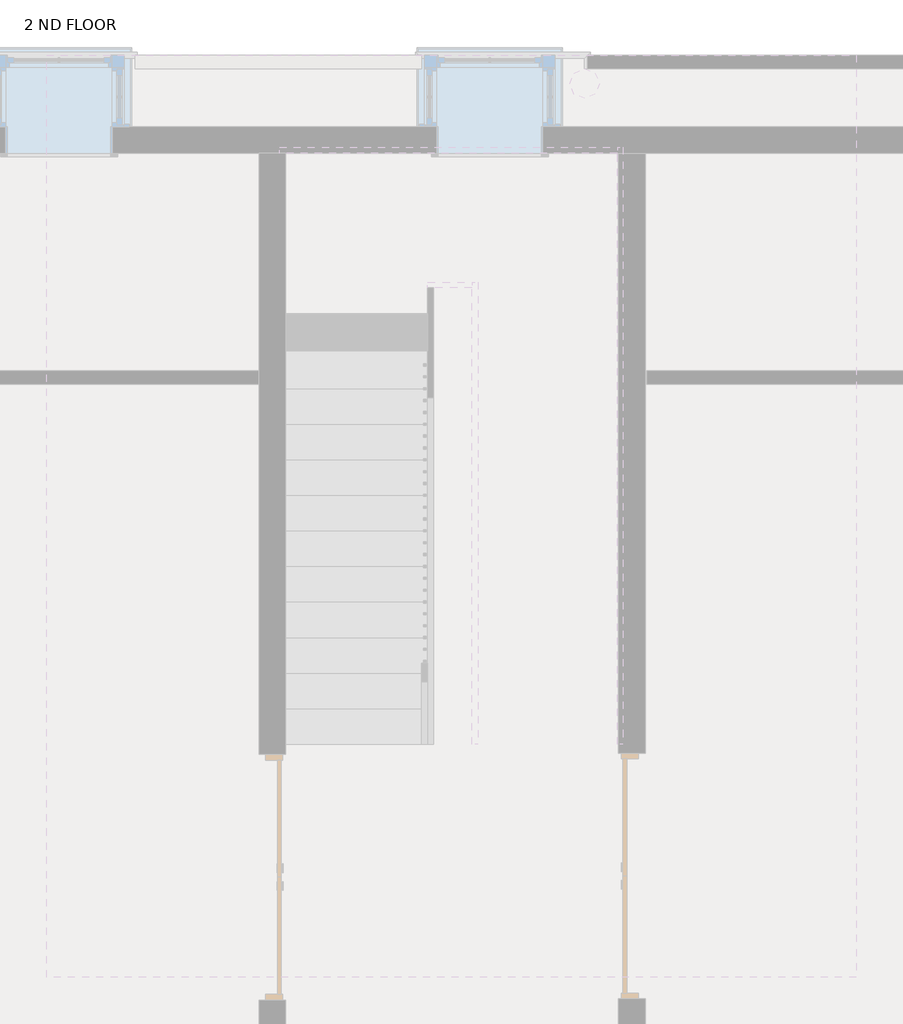
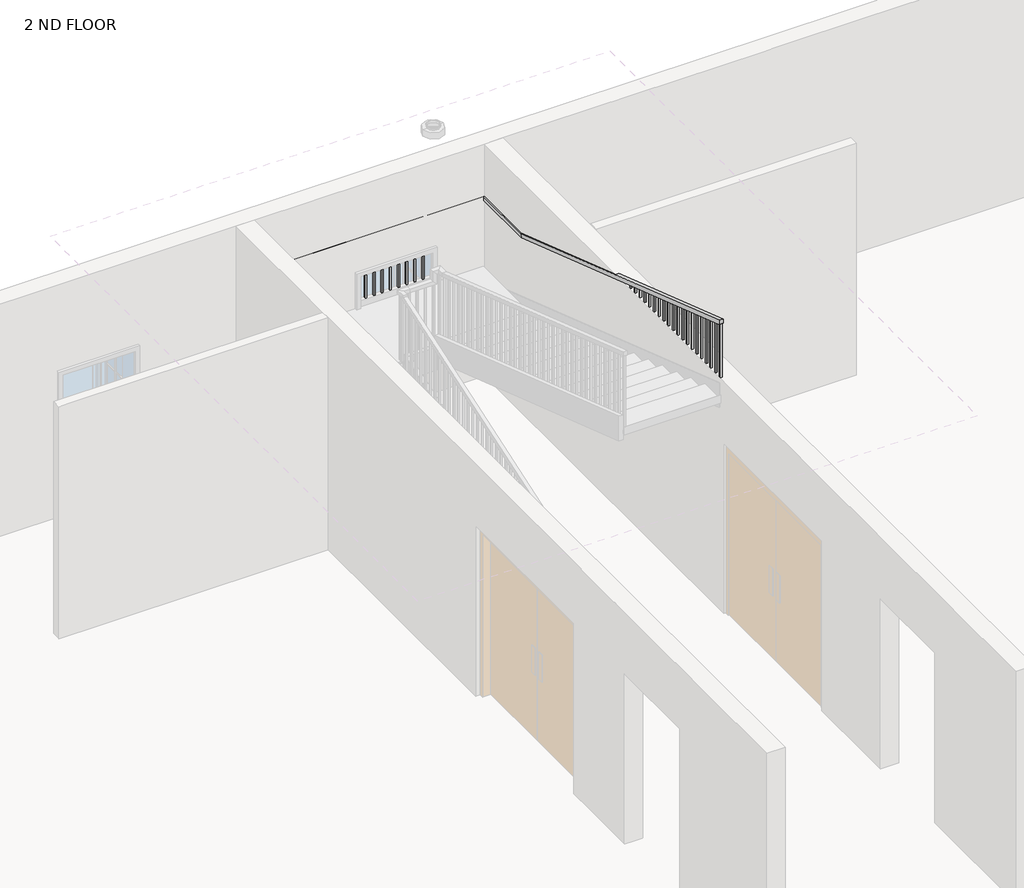
# One storey, part 5 of 7: 1 railing.
"""IFC4 building model written with IfcOpenShell, lengths in millimetres."""

from ifc_helpers import new_model, si_unit, frame, origin, place, context, project, spatial, polyline, outline, extrude, faceted_brep, element, save

model = new_model("IFC4")

# Units and contexts
model_context = context("Model", 3, world=origin())
ifc_project = project(units=[si_unit("LENGTHUNIT", "METRE", prefix="MILLI")], contexts=[model_context])

# Site, building, storey
site = spatial("IfcSite", under=ifc_project)
building = spatial("IfcBuilding", under=site)
storey = spatial("IfcBuildingStorey", under=building, Name="2 ND FLOOR", Elevation=6400.8)

# Railing
placement = place(None, origin())
element("IfcRailing", 1, ObjectType="Handrail - Rectangular", at=placement, inside=storey, context=model_context, shape_type="SolidModel", body=[
    faceted_brep([(-1899.5987998, 2564.5067329, 7418.6142857), (-1899.5987998, 2564.5067329, 7364.9699957), (-1848.7987998, 2564.5067329, 7364.9699957), (-1848.7987998, 2564.5067329, 7418.6142857), (-1899.5987998, 6526.9067329, 8763.0), (-1899.5987998, 6535.2899033, 8712.2), (-1848.7987998, 6535.2899033, 8712.2), (-1848.7987998, 6526.9067329, 8763.0), (-1899.5987998, 7682.6067329, 8712.2), (-1899.5987998, 7682.6067329, 8763.0), (1046.8012002, 7682.6067329, 8763.0), (1046.8012002, 7682.6067329, 8712.2), (-1848.7987998, 7631.8067329, 8712.2), (996.0012002, 7631.8067329, 8712.2), (-1848.7987998, 7631.8067329, 8763.0), (996.0012002, 7631.8067329, 8763.0), (1046.8012002, 6831.7067329, 8763.0), (1046.8012002, 6823.3235624, 8712.2), (996.0012002, 6823.3235624, 8712.2), (996.0012002, 6831.7067329, 8763.0), (1046.8012002, 2564.5067329, 10210.8), (996.0012002, 2564.5067329, 10210.8), (996.0012002, 2564.5067329, 10157.15571), (1046.8012002, 2564.5067329, 10157.15571)], [[[0, 1, 2, 3]], [[1, 0, 4, 5]], [[2, 1, 5, 6]], [[3, 2, 6, 7]], [[0, 3, 7, 4]], [[8, 9, 10, 11]], [[12, 8, 11, 13]], [[14, 12, 13, 15]], [[9, 14, 15, 10]], [[11, 10, 16, 17]], [[13, 11, 17, 18]], [[15, 13, 18, 19]], [[10, 15, 19, 16]], [[5, 4, 9, 8]], [[6, 5, 8, 12]], [[7, 6, 12, 14]], [[4, 7, 14, 9]], [[20, 21, 22, 23]], [[17, 16, 20, 23]], [[18, 17, 23, 22]], [[19, 18, 22, 21]], [[16, 19, 21, 20]]]),
    extrude(outline(polyline([(2586.7317329, 10149.615085), (2586.7317329, 9378.6831452), (2567.6817329, 9385.1465381), (2567.6817329, 10156.0784779), (2586.7317329, 10149.615085)])), frame((1011.8762002, 0.0, 0.0), z_axis=(1.0, 0.0, 0.0), x_axis=(0.0, 1.0, 0.0)), (0.0, 0.0, 1.0), 19.05),
    extrude(outline(polyline([(2688.3317329, 10115.1436565), (2688.3317329, 9344.2117167), (2669.2817329, 9350.6751095), (2669.2817329, 10121.6070493), (2688.3317329, 10115.1436565)])), frame((1011.8762002, 0.0, 0.0), z_axis=(1.0, 0.0, 0.0), x_axis=(0.0, 1.0, 0.0)), (0.0, 0.0, 1.0), 19.05),
    extrude(outline(polyline([(2789.9317329, 10080.6722279), (2789.9317329, 9309.7402881), (2770.8817329, 9316.203681), (2770.8817329, 10087.1356207), (2789.9317329, 10080.6722279)])), frame((1011.8762002, 0.0, 0.0), z_axis=(1.0, 0.0, 0.0), x_axis=(0.0, 1.0, 0.0)), (0.0, 0.0, 1.0), 19.05),
    extrude(outline(polyline([(2891.5317329, 10046.2007993), (2891.5317329, 9275.2688595), (2872.4817329, 9281.7322524), (2872.4817329, 10052.6641922), (2891.5317329, 10046.2007993)])), frame((1011.8762002, 0.0, 0.0), z_axis=(1.0, 0.0, 0.0), x_axis=(0.0, 1.0, 0.0)), (0.0, 0.0, 1.0), 19.05),
    extrude(outline(polyline([(2993.1317329, 10011.7293707), (2993.1317329, 9240.797431), (2974.0817329, 9247.2608238), (2974.0817329, 10018.1927636), (2993.1317329, 10011.7293707)])), frame((1011.8762002, 0.0, 0.0), z_axis=(1.0, 0.0, 0.0), x_axis=(0.0, 1.0, 0.0)), (0.0, 0.0, 1.0), 19.05),
    extrude(outline(polyline([(3094.7317329, 9977.2579422), (3094.7317329, 9206.3260024), (3075.6817329, 9212.7893952), (3075.6817329, 9983.721335), (3094.7317329, 9977.2579422)])), frame((1011.8762002, 0.0, 0.0), z_axis=(1.0, 0.0, 0.0), x_axis=(0.0, 1.0, 0.0)), (0.0, 0.0, 1.0), 19.05),
    extrude(outline(polyline([(3196.3317329, 9942.7865136), (3196.3317329, 9171.8545738), (3177.2817329, 9178.3179667), (3177.2817329, 9949.2499065), (3196.3317329, 9942.7865136)])), frame((1011.8762002, 0.0, 0.0), z_axis=(1.0, 0.0, 0.0), x_axis=(0.0, 1.0, 0.0)), (0.0, 0.0, 1.0), 19.05),
    extrude(outline(polyline([(3297.9317329, 9908.315085), (3297.9317329, 9137.3831452), (3278.8817329, 9143.8465381), (3278.8817329, 9914.7784779), (3297.9317329, 9908.315085)])), frame((1011.8762002, 0.0, 0.0), z_axis=(1.0, 0.0, 0.0), x_axis=(0.0, 1.0, 0.0)), (0.0, 0.0, 1.0), 19.05),
    extrude(outline(polyline([(3399.5317329, 9873.8436565), (3399.5317329, 9102.9117167), (3380.4817329, 9109.3751095), (3380.4817329, 9880.3070493), (3399.5317329, 9873.8436565)])), frame((1011.8762002, 0.0, 0.0), z_axis=(1.0, 0.0, 0.0), x_axis=(0.0, 1.0, 0.0)), (0.0, 0.0, 1.0), 19.05),
    extrude(outline(polyline([(3501.1317329, 9839.3722279), (3501.1317329, 9068.4402881), (3482.0817329, 9074.903681), (3482.0817329, 9845.8356207), (3501.1317329, 9839.3722279)])), frame((1011.8762002, 0.0, 0.0), z_axis=(1.0, 0.0, 0.0), x_axis=(0.0, 1.0, 0.0)), (0.0, 0.0, 1.0), 19.05),
    extrude(outline(polyline([(3602.7317329, 9804.9007993), (3602.7317329, 9033.9688595), (3583.6817329, 9040.4322524), (3583.6817329, 9811.3641922), (3602.7317329, 9804.9007993)])), frame((1011.8762002, 0.0, 0.0), z_axis=(1.0, 0.0, 0.0), x_axis=(0.0, 1.0, 0.0)), (0.0, 0.0, 1.0), 19.05),
    extrude(outline(polyline([(3704.3317329, 9770.4293707), (3704.3317329, 8999.497431), (3685.2817329, 9005.9608238), (3685.2817329, 9776.8927636), (3704.3317329, 9770.4293707)])), frame((1011.8762002, 0.0, 0.0), z_axis=(1.0, 0.0, 0.0), x_axis=(0.0, 1.0, 0.0)), (0.0, 0.0, 1.0), 19.05),
    extrude(outline(polyline([(3805.9317329, 9735.9579422), (3805.9317329, 8965.0260024), (3786.8817329, 8971.4893952), (3786.8817329, 9742.421335), (3805.9317329, 9735.9579422)])), frame((1011.8762002, 0.0, 0.0), z_axis=(1.0, 0.0, 0.0), x_axis=(0.0, 1.0, 0.0)), (0.0, 0.0, 1.0), 19.05),
    extrude(outline(polyline([(3907.5317329, 9701.4865136), (3907.5317329, 8930.5545738), (3888.4817329, 8937.0179667), (3888.4817329, 9707.9499065), (3907.5317329, 9701.4865136)])), frame((1011.8762002, 0.0, 0.0), z_axis=(1.0, 0.0, 0.0), x_axis=(0.0, 1.0, 0.0)), (0.0, 0.0, 1.0), 19.05),
    extrude(outline(polyline([(4009.1317329, 9667.015085), (4009.1317329, 8896.0831452), (3990.0817329, 8902.5465381), (3990.0817329, 9673.4784779), (4009.1317329, 9667.015085)])), frame((1011.8762002, 0.0, 0.0), z_axis=(1.0, 0.0, 0.0), x_axis=(0.0, 1.0, 0.0)), (0.0, 0.0, 1.0), 19.05),
    extrude(outline(polyline([(4110.7317329, 9632.5436565), (4110.7317329, 8861.6117167), (4091.6817329, 8868.0751095), (4091.6817329, 9639.0070493), (4110.7317329, 9632.5436565)])), frame((1011.8762002, 0.0, 0.0), z_axis=(1.0, 0.0, 0.0), x_axis=(0.0, 1.0, 0.0)), (0.0, 0.0, 1.0), 19.05),
    extrude(outline(polyline([(4212.3317329, 9598.0722279), (4212.3317329, 8827.1402881), (4193.2817329, 8833.603681), (4193.2817329, 9604.5356207), (4212.3317329, 9598.0722279)])), frame((1011.8762002, 0.0, 0.0), z_axis=(1.0, 0.0, 0.0), x_axis=(0.0, 1.0, 0.0)), (0.0, 0.0, 1.0), 19.05),
    extrude(outline(polyline([(4313.9317329, 9563.6007993), (4313.9317329, 8792.6688595), (4294.8817329, 8799.1322524), (4294.8817329, 9570.0641922), (4313.9317329, 9563.6007993)])), frame((1011.8762002, 0.0, 0.0), z_axis=(1.0, 0.0, 0.0), x_axis=(0.0, 1.0, 0.0)), (0.0, 0.0, 1.0), 19.05),
    extrude(outline(polyline([(4415.5317329, 9529.1293707), (4415.5317329, 8758.197431), (4396.4817329, 8764.6608238), (4396.4817329, 9535.5927636), (4415.5317329, 9529.1293707)])), frame((1011.8762002, 0.0, 0.0), z_axis=(1.0, 0.0, 0.0), x_axis=(0.0, 1.0, 0.0)), (0.0, 0.0, 1.0), 19.05),
    extrude(outline(polyline([(4517.1317329, 9494.6579422), (4517.1317329, 8723.7260024), (4498.0817329, 8730.1893952), (4498.0817329, 9501.121335), (4517.1317329, 9494.6579422)])), frame((1011.8762002, 0.0, 0.0), z_axis=(1.0, 0.0, 0.0), x_axis=(0.0, 1.0, 0.0)), (0.0, 0.0, 1.0), 19.05),
    extrude(outline(polyline([(4618.7317329, 9460.1865136), (4618.7317329, 8689.2545738), (4599.6817329, 8695.7179667), (4599.6817329, 9466.6499065), (4618.7317329, 9460.1865136)])), frame((1011.8762002, 0.0, 0.0), z_axis=(1.0, 0.0, 0.0), x_axis=(0.0, 1.0, 0.0)), (0.0, 0.0, 1.0), 19.05),
    extrude(outline(polyline([(4720.3317329, 9425.715085), (4720.3317329, 8654.7831452), (4701.2817329, 8661.2465381), (4701.2817329, 9432.1784779), (4720.3317329, 9425.715085)])), frame((1011.8762002, 0.0, 0.0), z_axis=(1.0, 0.0, 0.0), x_axis=(0.0, 1.0, 0.0)), (0.0, 0.0, 1.0), 19.05),
    extrude(outline(polyline([(4821.9317329, 9391.2436565), (4821.9317329, 8620.3117167), (4802.8817329, 8626.7751095), (4802.8817329, 9397.7070493), (4821.9317329, 9391.2436565)])), frame((1011.8762002, 0.0, 0.0), z_axis=(1.0, 0.0, 0.0), x_axis=(0.0, 1.0, 0.0)), (0.0, 0.0, 1.0), 19.05),
    extrude(outline(polyline([(4923.5317329, 9356.7722279), (4923.5317329, 8585.8402881), (4904.4817329, 8592.303681), (4904.4817329, 9363.2356207), (4923.5317329, 9356.7722279)])), frame((1011.8762002, 0.0, 0.0), z_axis=(1.0, 0.0, 0.0), x_axis=(0.0, 1.0, 0.0)), (0.0, 0.0, 1.0), 19.05),
    extrude(outline(polyline([(5025.1317329, 9322.3007993), (5025.1317329, 8551.3688595), (5006.0817329, 8557.8322524), (5006.0817329, 9328.7641922), (5025.1317329, 9322.3007993)])), frame((1011.8762002, 0.0, 0.0), z_axis=(1.0, 0.0, 0.0), x_axis=(0.0, 1.0, 0.0)), (0.0, 0.0, 1.0), 19.05),
    extrude(outline(polyline([(5126.7317329, 9287.8293707), (5126.7317329, 8516.897431), (5107.6817329, 8523.3608238), (5107.6817329, 9294.2927636), (5126.7317329, 9287.8293707)])), frame((1011.8762002, 0.0, 0.0), z_axis=(1.0, 0.0, 0.0), x_axis=(0.0, 1.0, 0.0)), (0.0, 0.0, 1.0), 19.05),
    extrude(outline(polyline([(5228.3317329, 9253.3579422), (5228.3317329, 8482.4260024), (5209.2817329, 8488.8893952), (5209.2817329, 9259.821335), (5228.3317329, 9253.3579422)])), frame((1011.8762002, 0.0, 0.0), z_axis=(1.0, 0.0, 0.0), x_axis=(0.0, 1.0, 0.0)), (0.0, 0.0, 1.0), 19.05),
    extrude(outline(polyline([(5329.9317329, 9218.8865136), (5329.9317329, 8447.9545738), (5310.8817329, 8454.4179667), (5310.8817329, 9225.3499065), (5329.9317329, 9218.8865136)])), frame((1011.8762002, 0.0, 0.0), z_axis=(1.0, 0.0, 0.0), x_axis=(0.0, 1.0, 0.0)), (0.0, 0.0, 1.0), 19.05),
    extrude(outline(polyline([(5431.5317329, 9184.415085), (5431.5317329, 8413.4831452), (5412.4817329, 8419.9465381), (5412.4817329, 9190.8784779), (5431.5317329, 9184.415085)])), frame((1011.8762002, 0.0, 0.0), z_axis=(1.0, 0.0, 0.0), x_axis=(0.0, 1.0, 0.0)), (0.0, 0.0, 1.0), 19.05),
    extrude(outline(polyline([(5533.1317329, 9149.9436565), (5533.1317329, 8379.0117167), (5514.0817329, 8385.4751095), (5514.0817329, 9156.4070493), (5533.1317329, 9149.9436565)])), frame((1011.8762002, 0.0, 0.0), z_axis=(1.0, 0.0, 0.0), x_axis=(0.0, 1.0, 0.0)), (0.0, 0.0, 1.0), 19.05),
    extrude(outline(polyline([(5634.7317329, 9115.4722279), (5634.7317329, 8344.5402881), (5615.6817329, 8351.003681), (5615.6817329, 9121.9356207), (5634.7317329, 9115.4722279)])), frame((1011.8762002, 0.0, 0.0), z_axis=(1.0, 0.0, 0.0), x_axis=(0.0, 1.0, 0.0)), (0.0, 0.0, 1.0), 19.05),
    extrude(outline(polyline([(5736.3317329, 9081.0007993), (5736.3317329, 8310.0688595), (5717.2817329, 8316.5322524), (5717.2817329, 9087.4641922), (5736.3317329, 9081.0007993)])), frame((1011.8762002, 0.0, 0.0), z_axis=(1.0, 0.0, 0.0), x_axis=(0.0, 1.0, 0.0)), (0.0, 0.0, 1.0), 19.05),
    extrude(outline(polyline([(5837.9317329, 9046.5293707), (5837.9317329, 8275.597431), (5818.8817329, 8282.0608238), (5818.8817329, 9052.9927636), (5837.9317329, 9046.5293707)])), frame((1011.8762002, 0.0, 0.0), z_axis=(1.0, 0.0, 0.0), x_axis=(0.0, 1.0, 0.0)), (0.0, 0.0, 1.0), 19.05),
    extrude(outline(polyline([(5939.5317329, 9012.0579422), (5939.5317329, 8241.1260024), (5920.4817329, 8247.5893952), (5920.4817329, 9018.521335), (5939.5317329, 9012.0579422)])), frame((1011.8762002, 0.0, 0.0), z_axis=(1.0, 0.0, 0.0), x_axis=(0.0, 1.0, 0.0)), (0.0, 0.0, 1.0), 19.05),
    extrude(outline(polyline([(6041.1317329, 8977.5865136), (6041.1317329, 8206.6545738), (6022.0817329, 8213.1179667), (6022.0817329, 8984.0499065), (6041.1317329, 8977.5865136)])), frame((1011.8762002, 0.0, 0.0), z_axis=(1.0, 0.0, 0.0), x_axis=(0.0, 1.0, 0.0)), (0.0, 0.0, 1.0), 19.05),
    extrude(outline(polyline([(6142.7317329, 8943.115085), (6142.7317329, 8172.1831452), (6123.6817329, 8178.6465381), (6123.6817329, 8949.5784779), (6142.7317329, 8943.115085)])), frame((1011.8762002, 0.0, 0.0), z_axis=(1.0, 0.0, 0.0), x_axis=(0.0, 1.0, 0.0)), (0.0, 0.0, 1.0), 19.05),
    extrude(outline(polyline([(6244.3317329, 8908.6436565), (6244.3317329, 8137.7117167), (6225.2817329, 8144.1751095), (6225.2817329, 8915.1070493), (6244.3317329, 8908.6436565)])), frame((1011.8762002, 0.0, 0.0), z_axis=(1.0, 0.0, 0.0), x_axis=(0.0, 1.0, 0.0)), (0.0, 0.0, 1.0), 19.05),
    extrude(outline(polyline([(6345.9317329, 8874.1722279), (6345.9317329, 8103.2402881), (6326.8817329, 8109.703681), (6326.8817329, 8880.6356207), (6345.9317329, 8874.1722279)])), frame((1011.8762002, 0.0, 0.0), z_axis=(1.0, 0.0, 0.0), x_axis=(0.0, 1.0, 0.0)), (0.0, 0.0, 1.0), 19.05),
    extrude(outline(polyline([(6447.5317329, 8839.7007993), (6447.5317329, 8068.7688595), (6428.4817329, 8075.2322524), (6428.4817329, 8846.1641922), (6447.5317329, 8839.7007993)])), frame((1011.8762002, 0.0, 0.0), z_axis=(1.0, 0.0, 0.0), x_axis=(0.0, 1.0, 0.0)), (0.0, 0.0, 1.0), 19.05),
    extrude(outline(polyline([(6549.1317329, 8805.2293707), (6549.1317329, 8034.297431), (6530.0817329, 8040.7608238), (6530.0817329, 8811.6927636), (6549.1317329, 8805.2293707)])), frame((1011.8762002, 0.0, 0.0), z_axis=(1.0, 0.0, 0.0), x_axis=(0.0, 1.0, 0.0)), (0.0, 0.0, 1.0), 19.05),
    extrude(outline(polyline([(6650.7317329, 8770.7579422), (6650.7317329, 7999.8260024), (6631.6817329, 8006.2893952), (6631.6817329, 8777.221335), (6650.7317329, 8770.7579422)])), frame((1011.8762002, 0.0, 0.0), z_axis=(1.0, 0.0, 0.0), x_axis=(0.0, 1.0, 0.0)), (0.0, 0.0, 1.0), 19.05),
    extrude(outline(polyline([(6752.3317329, 8736.2865136), (6752.3317329, 7965.3545738), (6733.2817329, 7971.8179667), (6733.2817329, 8742.7499065), (6752.3317329, 8736.2865136)])), frame((1011.8762002, 0.0, 0.0), z_axis=(1.0, 0.0, 0.0), x_axis=(0.0, 1.0, 0.0)), (0.0, 0.0, 1.0), 19.05),
    extrude(outline(polyline([(6853.9317329, 8712.2), (6853.9317329, 7930.8831452), (6834.8817329, 7937.3465381), (6834.8817329, 8712.2), (6853.9317329, 8712.2)])), frame((1011.8762002, 0.0, 0.0), z_axis=(1.0, 0.0, 0.0), x_axis=(0.0, 1.0, 0.0)), (0.0, 0.0, 1.0), 19.05),
    extrude(outline(polyline([(6955.5317329, 8712.2), (6955.5317329, 7896.4117167), (6936.4817329, 7902.8751095), (6936.4817329, 8712.2), (6955.5317329, 8712.2)])), frame((1011.8762002, 0.0, 0.0), z_axis=(1.0, 0.0, 0.0), x_axis=(0.0, 1.0, 0.0)), (0.0, 0.0, 1.0), 19.05),
    extrude(outline(polyline([(7057.1317329, 8712.2), (7057.1317329, 7861.9402881), (7038.0817329, 7868.403681), (7038.0817329, 8712.2), (7057.1317329, 8712.2)])), frame((1011.8762002, 0.0, 0.0), z_axis=(1.0, 0.0, 0.0), x_axis=(0.0, 1.0, 0.0)), (0.0, 0.0, 1.0), 19.05),
    extrude(outline(polyline([(7158.7317329, 8712.2), (7158.7317329, 7827.4688595), (7139.6817329, 7833.9322524), (7139.6817329, 8712.2), (7158.7317329, 8712.2)])), frame((1011.8762002, 0.0, 0.0), z_axis=(1.0, 0.0, 0.0), x_axis=(0.0, 1.0, 0.0)), (0.0, 0.0, 1.0), 19.05),
    extrude(outline(polyline([(7260.3317329, 8712.2), (7260.3317329, 7792.997431), (7241.2817329, 7799.4608238), (7241.2817329, 8712.2), (7260.3317329, 8712.2)])), frame((1011.8762002, 0.0, 0.0), z_axis=(1.0, 0.0, 0.0), x_axis=(0.0, 1.0, 0.0)), (0.0, 0.0, 1.0), 19.05),
    extrude(outline(polyline([(7361.9317329, 8712.2), (7361.9317329, 7758.5260024), (7342.8817329, 7764.9893952), (7342.8817329, 8712.2), (7361.9317329, 8712.2)])), frame((1011.8762002, 0.0, 0.0), z_axis=(1.0, 0.0, 0.0), x_axis=(0.0, 1.0, 0.0)), (0.0, 0.0, 1.0), 19.05),
    extrude(outline(polyline([(7463.5317329, 8712.2), (7463.5317329, 7724.0545738), (7444.4817329, 7730.5179667), (7444.4817329, 8712.2), (7463.5317329, 8712.2)])), frame((1011.8762002, 0.0, 0.0), z_axis=(1.0, 0.0, 0.0), x_axis=(0.0, 1.0, 0.0)), (0.0, 0.0, 1.0), 19.05),
    extrude(outline(polyline([(7565.1317329, 8712.2), (7565.1317329, 7689.5831452), (7546.0817329, 7696.0465381), (7546.0817329, 8712.2), (7565.1317329, 8712.2)])), frame((1011.8762002, 0.0, 0.0), z_axis=(1.0, 0.0, 0.0), x_axis=(0.0, 1.0, 0.0)), (0.0, 0.0, 1.0), 19.05),
    extrude(outline(polyline([(961.0762002, 7666.7317329), (980.1262002, 7666.7317329), (980.1262002, 7647.6817329), (961.0762002, 7647.6817329), (961.0762002, 7666.7317329)])), frame((0.0, 0.0, 7924.8), z_axis=(0.0, 0.0, 1.0), x_axis=(1.0, 0.0, 0.0)), (0.0, 0.0, 1.0), 787.4),
    extrude(outline(polyline([(859.4762002, 7666.7317329), (878.5262002, 7666.7317329), (878.5262002, 7647.6817329), (859.4762002, 7647.6817329), (859.4762002, 7666.7317329)])), frame((0.0, 0.0, 7924.8), z_axis=(0.0, 0.0, 1.0), x_axis=(1.0, 0.0, 0.0)), (0.0, 0.0, 1.0), 787.4),
    extrude(outline(polyline([(757.8762002, 7666.7317329), (776.9262002, 7666.7317329), (776.9262002, 7647.6817329), (757.8762002, 7647.6817329), (757.8762002, 7666.7317329)])), frame((0.0, 0.0, 7924.8), z_axis=(0.0, 0.0, 1.0), x_axis=(1.0, 0.0, 0.0)), (0.0, 0.0, 1.0), 787.4),
    extrude(outline(polyline([(656.2762002, 7666.7317329), (675.3262002, 7666.7317329), (675.3262002, 7647.6817329), (656.2762002, 7647.6817329), (656.2762002, 7666.7317329)])), frame((0.0, 0.0, 7924.8), z_axis=(0.0, 0.0, 1.0), x_axis=(1.0, 0.0, 0.0)), (0.0, 0.0, 1.0), 787.4),
    extrude(outline(polyline([(554.6762002, 7666.7317329), (573.7262002, 7666.7317329), (573.7262002, 7647.6817329), (554.6762002, 7647.6817329), (554.6762002, 7666.7317329)])), frame((0.0, 0.0, 7924.8), z_axis=(0.0, 0.0, 1.0), x_axis=(1.0, 0.0, 0.0)), (0.0, 0.0, 1.0), 787.4),
    extrude(outline(polyline([(453.0762002, 7666.7317329), (472.1262002, 7666.7317329), (472.1262002, 7647.6817329), (453.0762002, 7647.6817329), (453.0762002, 7666.7317329)])), frame((0.0, 0.0, 7924.8), z_axis=(0.0, 0.0, 1.0), x_axis=(1.0, 0.0, 0.0)), (0.0, 0.0, 1.0), 787.4),
    extrude(outline(polyline([(351.4762002, 7666.7317329), (370.5262002, 7666.7317329), (370.5262002, 7647.6817329), (351.4762002, 7647.6817329), (351.4762002, 7666.7317329)])), frame((0.0, 0.0, 7924.8), z_axis=(0.0, 0.0, 1.0), x_axis=(1.0, 0.0, 0.0)), (0.0, 0.0, 1.0), 787.4),
    extrude(outline(polyline([(249.8762002, 7666.7317329), (268.9262002, 7666.7317329), (268.9262002, 7647.6817329), (249.8762002, 7647.6817329), (249.8762002, 7666.7317329)])), frame((0.0, 0.0, 7924.8), z_axis=(0.0, 0.0, 1.0), x_axis=(1.0, 0.0, 0.0)), (0.0, 0.0, 1.0), 787.4),
    extrude(outline(polyline([(148.2762002, 7666.7317329), (167.3262002, 7666.7317329), (167.3262002, 7647.6817329), (148.2762002, 7647.6817329), (148.2762002, 7666.7317329)])), frame((0.0, 0.0, 7924.8), z_axis=(0.0, 0.0, 1.0), x_axis=(1.0, 0.0, 0.0)), (0.0, 0.0, 1.0), 787.4),
    extrude(outline(polyline([(46.6762002, 7666.7317329), (65.7262002, 7666.7317329), (65.7262002, 7647.6817329), (46.6762002, 7647.6817329), (46.6762002, 7666.7317329)])), frame((0.0, 0.0, 7924.8), z_axis=(0.0, 0.0, 1.0), x_axis=(1.0, 0.0, 0.0)), (0.0, 0.0, 1.0), 787.4),
    extrude(outline(polyline([(-54.9237998, 7666.7317329), (-35.8737998, 7666.7317329), (-35.8737998, 7647.6817329), (-54.9237998, 7647.6817329), (-54.9237998, 7666.7317329)])), frame((0.0, 0.0, 7924.8), z_axis=(0.0, 0.0, 1.0), x_axis=(1.0, 0.0, 0.0)), (0.0, 0.0, 1.0), 787.4),
    extrude(outline(polyline([(-156.5237998, 7666.7317329), (-137.4737998, 7666.7317329), (-137.4737998, 7647.6817329), (-156.5237998, 7647.6817329), (-156.5237998, 7666.7317329)])), frame((0.0, 0.0, 7924.8), z_axis=(0.0, 0.0, 1.0), x_axis=(1.0, 0.0, 0.0)), (0.0, 0.0, 1.0), 787.4),
    extrude(outline(polyline([(-258.1237998, 7666.7317329), (-239.0737998, 7666.7317329), (-239.0737998, 7647.6817329), (-258.1237998, 7647.6817329), (-258.1237998, 7666.7317329)])), frame((0.0, 0.0, 7924.8), z_axis=(0.0, 0.0, 1.0), x_axis=(1.0, 0.0, 0.0)), (0.0, 0.0, 1.0), 787.4),
    extrude(outline(polyline([(-359.7237998, 7666.7317329), (-340.6737998, 7666.7317329), (-340.6737998, 7647.6817329), (-359.7237998, 7647.6817329), (-359.7237998, 7666.7317329)])), frame((0.0, 0.0, 7924.8), z_axis=(0.0, 0.0, 1.0), x_axis=(1.0, 0.0, 0.0)), (0.0, 0.0, 1.0), 787.4),
    extrude(outline(polyline([(-461.3237998, 7666.7317329), (-442.2737998, 7666.7317329), (-442.2737998, 7647.6817329), (-461.3237998, 7647.6817329), (-461.3237998, 7666.7317329)])), frame((0.0, 0.0, 7924.8), z_axis=(0.0, 0.0, 1.0), x_axis=(1.0, 0.0, 0.0)), (0.0, 0.0, 1.0), 787.4),
    extrude(outline(polyline([(-562.9237998, 7666.7317329), (-543.8737998, 7666.7317329), (-543.8737998, 7647.6817329), (-562.9237998, 7647.6817329), (-562.9237998, 7666.7317329)])), frame((0.0, 0.0, 7924.8), z_axis=(0.0, 0.0, 1.0), x_axis=(1.0, 0.0, 0.0)), (0.0, 0.0, 1.0), 787.4),
    extrude(outline(polyline([(-664.5237998, 7666.7317329), (-645.4737998, 7666.7317329), (-645.4737998, 7647.6817329), (-664.5237998, 7647.6817329), (-664.5237998, 7666.7317329)])), frame((0.0, 0.0, 7924.8), z_axis=(0.0, 0.0, 1.0), x_axis=(1.0, 0.0, 0.0)), (0.0, 0.0, 1.0), 787.4),
    extrude(outline(polyline([(-766.1237998, 7666.7317329), (-747.0737998, 7666.7317329), (-747.0737998, 7647.6817329), (-766.1237998, 7647.6817329), (-766.1237998, 7666.7317329)])), frame((0.0, 0.0, 7924.8), z_axis=(0.0, 0.0, 1.0), x_axis=(1.0, 0.0, 0.0)), (0.0, 0.0, 1.0), 787.4),
    extrude(outline(polyline([(-867.7237998, 7666.7317329), (-848.6737998, 7666.7317329), (-848.6737998, 7647.6817329), (-867.7237998, 7647.6817329), (-867.7237998, 7666.7317329)])), frame((0.0, 0.0, 7924.8), z_axis=(0.0, 0.0, 1.0), x_axis=(1.0, 0.0, 0.0)), (0.0, 0.0, 1.0), 787.4),
    extrude(outline(polyline([(-969.3237998, 7666.7317329), (-950.2737998, 7666.7317329), (-950.2737998, 7647.6817329), (-969.3237998, 7647.6817329), (-969.3237998, 7666.7317329)])), frame((0.0, 0.0, 7924.8), z_axis=(0.0, 0.0, 1.0), x_axis=(1.0, 0.0, 0.0)), (0.0, 0.0, 1.0), 787.4),
    extrude(outline(polyline([(-1070.9237998, 7666.7317329), (-1051.8737998, 7666.7317329), (-1051.8737998, 7647.6817329), (-1070.9237998, 7647.6817329), (-1070.9237998, 7666.7317329)])), frame((0.0, 0.0, 7924.8), z_axis=(0.0, 0.0, 1.0), x_axis=(1.0, 0.0, 0.0)), (0.0, 0.0, 1.0), 787.4),
    extrude(outline(polyline([(-1172.5237998, 7666.7317329), (-1153.4737998, 7666.7317329), (-1153.4737998, 7647.6817329), (-1172.5237998, 7647.6817329), (-1172.5237998, 7666.7317329)])), frame((0.0, 0.0, 7924.8), z_axis=(0.0, 0.0, 1.0), x_axis=(1.0, 0.0, 0.0)), (0.0, 0.0, 1.0), 787.4),
    extrude(outline(polyline([(-1274.1237998, 7666.7317329), (-1255.0737998, 7666.7317329), (-1255.0737998, 7647.6817329), (-1274.1237998, 7647.6817329), (-1274.1237998, 7666.7317329)])), frame((0.0, 0.0, 7924.8), z_axis=(0.0, 0.0, 1.0), x_axis=(1.0, 0.0, 0.0)), (0.0, 0.0, 1.0), 787.4),
    extrude(outline(polyline([(-1375.7237998, 7666.7317329), (-1356.6737998, 7666.7317329), (-1356.6737998, 7647.6817329), (-1375.7237998, 7647.6817329), (-1375.7237998, 7666.7317329)])), frame((0.0, 0.0, 7924.8), z_axis=(0.0, 0.0, 1.0), x_axis=(1.0, 0.0, 0.0)), (0.0, 0.0, 1.0), 787.4),
    extrude(outline(polyline([(-1477.3237998, 7666.7317329), (-1458.2737998, 7666.7317329), (-1458.2737998, 7647.6817329), (-1477.3237998, 7647.6817329), (-1477.3237998, 7666.7317329)])), frame((0.0, 0.0, 7924.8), z_axis=(0.0, 0.0, 1.0), x_axis=(1.0, 0.0, 0.0)), (0.0, 0.0, 1.0), 787.4),
    extrude(outline(polyline([(-1578.9237998, 7666.7317329), (-1559.8737998, 7666.7317329), (-1559.8737998, 7647.6817329), (-1578.9237998, 7647.6817329), (-1578.9237998, 7666.7317329)])), frame((0.0, 0.0, 7924.8), z_axis=(0.0, 0.0, 1.0), x_axis=(1.0, 0.0, 0.0)), (0.0, 0.0, 1.0), 787.4),
    extrude(outline(polyline([(-1680.5237998, 7666.7317329), (-1661.4737998, 7666.7317329), (-1661.4737998, 7647.6817329), (-1680.5237998, 7647.6817329), (-1680.5237998, 7666.7317329)])), frame((0.0, 0.0, 7924.8), z_axis=(0.0, 0.0, 1.0), x_axis=(1.0, 0.0, 0.0)), (0.0, 0.0, 1.0), 787.4),
    extrude(outline(polyline([(-1782.1237998, 7666.7317329), (-1763.0737998, 7666.7317329), (-1763.0737998, 7647.6817329), (-1782.1237998, 7647.6817329), (-1782.1237998, 7666.7317329)])), frame((0.0, 0.0, 7924.8), z_axis=(0.0, 0.0, 1.0), x_axis=(1.0, 0.0, 0.0)), (0.0, 0.0, 1.0), 787.4),
    extrude(outline(polyline([(-1883.7237998, 7634.9817329), (-1883.7237998, 7654.0317329), (-1864.6737998, 7654.0317329), (-1864.6737998, 7634.9817329), (-1883.7237998, 7634.9817329)])), frame((0.0, 0.0, 8227.7857143), z_axis=(0.0, 0.0, 1.0), x_axis=(1.0, 0.0, 0.0)), (0.0, 0.0, 1.0), 484.4142857),
    extrude(outline(polyline([(-1883.7237998, 7533.3817329), (-1883.7237998, 7552.4317329), (-1864.6737998, 7552.4317329), (-1864.6737998, 7533.3817329), (-1883.7237998, 7533.3817329)])), frame((0.0, 0.0, 8193.3142857), z_axis=(0.0, 0.0, 1.0), x_axis=(1.0, 0.0, 0.0)), (0.0, 0.0, 1.0), 518.8857143),
    extrude(outline(polyline([(-1883.7237998, 7431.7817329), (-1883.7237998, 7450.8317329), (-1864.6737998, 7450.8317329), (-1864.6737998, 7431.7817329), (-1883.7237998, 7431.7817329)])), frame((0.0, 0.0, 8158.8428571), z_axis=(0.0, 0.0, 1.0), x_axis=(1.0, 0.0, 0.0)), (0.0, 0.0, 1.0), 553.3571429),
    extrude(outline(polyline([(-1883.7237998, 7330.1817329), (-1883.7237998, 7349.2317329), (-1864.6737998, 7349.2317329), (-1864.6737998, 7330.1817329), (-1883.7237998, 7330.1817329)])), frame((0.0, 0.0, 8124.3714286), z_axis=(0.0, 0.0, 1.0), x_axis=(1.0, 0.0, 0.0)), (0.0, 0.0, 1.0), 587.8285714),
    extrude(outline(polyline([(-1883.7237998, 7228.5817329), (-1883.7237998, 7247.6317329), (-1864.6737998, 7247.6317329), (-1864.6737998, 7228.5817329), (-1883.7237998, 7228.5817329)])), frame((0.0, 0.0, 8089.9), z_axis=(0.0, 0.0, 1.0), x_axis=(1.0, 0.0, 0.0)), (0.0, 0.0, 1.0), 622.3),
    extrude(outline(polyline([(-1883.7237998, 7126.9817329), (-1883.7237998, 7146.0317329), (-1864.6737998, 7146.0317329), (-1864.6737998, 7126.9817329), (-1883.7237998, 7126.9817329)])), frame((0.0, 0.0, 8055.4285714), z_axis=(0.0, 0.0, 1.0), x_axis=(1.0, 0.0, 0.0)), (0.0, 0.0, 1.0), 656.7714286),
    extrude(outline(polyline([(-1883.7237998, 7025.3817329), (-1883.7237998, 7044.4317329), (-1864.6737998, 7044.4317329), (-1864.6737998, 7025.3817329), (-1883.7237998, 7025.3817329)])), frame((0.0, 0.0, 7924.8), z_axis=(0.0, 0.0, 1.0), x_axis=(1.0, 0.0, 0.0)), (0.0, 0.0, 1.0), 787.4),
    extrude(outline(polyline([(-1883.7237998, 6923.7817329), (-1883.7237998, 6942.8317329), (-1864.6737998, 6942.8317329), (-1864.6737998, 6923.7817329), (-1883.7237998, 6923.7817329)])), frame((0.0, 0.0, 7924.8), z_axis=(0.0, 0.0, 1.0), x_axis=(1.0, 0.0, 0.0)), (0.0, 0.0, 1.0), 787.4),
    extrude(outline(polyline([(-1883.7237998, 6822.1817329), (-1883.7237998, 6841.2317329), (-1864.6737998, 6841.2317329), (-1864.6737998, 6822.1817329), (-1883.7237998, 6822.1817329)])), frame((0.0, 0.0, 7924.8), z_axis=(0.0, 0.0, 1.0), x_axis=(1.0, 0.0, 0.0)), (0.0, 0.0, 1.0), 787.4),
    extrude(outline(polyline([(-1883.7237998, 6720.5817329), (-1883.7237998, 6739.6317329), (-1864.6737998, 6739.6317329), (-1864.6737998, 6720.5817329), (-1883.7237998, 6720.5817329)])), frame((0.0, 0.0, 7924.8), z_axis=(0.0, 0.0, 1.0), x_axis=(1.0, 0.0, 0.0)), (0.0, 0.0, 1.0), 787.4),
    extrude(outline(polyline([(-1883.7237998, 6618.9817329), (-1883.7237998, 6638.0317329), (-1864.6737998, 6638.0317329), (-1864.6737998, 6618.9817329), (-1883.7237998, 6618.9817329)])), frame((0.0, 0.0, 7924.8), z_axis=(0.0, 0.0, 1.0), x_axis=(1.0, 0.0, 0.0)), (0.0, 0.0, 1.0), 787.4),
    extrude(outline(polyline([(6536.4317329, 8712.5874065), (6536.4317329, 7924.8), (6517.3817329, 7924.8), (6517.3817329, 8706.1240136), (6536.4317329, 8712.5874065)])), frame((-1883.7237998, 0.0, 0.0), z_axis=(1.0, 0.0, 0.0), x_axis=(0.0, 1.0, 0.0)), (0.0, 0.0, 1.0), 19.05),
    extrude(outline(polyline([(6434.8317329, 8678.1159779), (6434.8317329, 7907.1840381), (6415.7817329, 7900.7206452), (6415.7817329, 8671.652585), (6434.8317329, 8678.1159779)])), frame((-1883.7237998, 0.0, 0.0), z_axis=(1.0, 0.0, 0.0), x_axis=(0.0, 1.0, 0.0)), (0.0, 0.0, 1.0), 19.05),
    extrude(outline(polyline([(6333.2317329, 8643.6445493), (6333.2317329, 7872.7126095), (6314.1817329, 7866.2492167), (6314.1817329, 8637.1811565), (6333.2317329, 8643.6445493)])), frame((-1883.7237998, 0.0, 0.0), z_axis=(1.0, 0.0, 0.0), x_axis=(0.0, 1.0, 0.0)), (0.0, 0.0, 1.0), 19.05),
    extrude(outline(polyline([(6231.6317329, 8609.1731207), (6231.6317329, 7838.241181), (6212.5817329, 7831.7777881), (6212.5817329, 8602.7097279), (6231.6317329, 8609.1731207)])), frame((-1883.7237998, 0.0, 0.0), z_axis=(1.0, 0.0, 0.0), x_axis=(0.0, 1.0, 0.0)), (0.0, 0.0, 1.0), 19.05),
    extrude(outline(polyline([(6130.0317329, 8574.7016922), (6130.0317329, 7803.7697524), (6110.9817329, 7797.3063595), (6110.9817329, 8568.2382993), (6130.0317329, 8574.7016922)])), frame((-1883.7237998, 0.0, 0.0), z_axis=(1.0, 0.0, 0.0), x_axis=(0.0, 1.0, 0.0)), (0.0, 0.0, 1.0), 19.05),
    extrude(outline(polyline([(6028.4317329, 8540.2302636), (6028.4317329, 7769.2983238), (6009.3817329, 7762.834931), (6009.3817329, 8533.7668707), (6028.4317329, 8540.2302636)])), frame((-1883.7237998, 0.0, 0.0), z_axis=(1.0, 0.0, 0.0), x_axis=(0.0, 1.0, 0.0)), (0.0, 0.0, 1.0), 19.05),
    extrude(outline(polyline([(5926.8317329, 8505.758835), (5926.8317329, 7734.8268952), (5907.7817329, 7728.3635024), (5907.7817329, 8499.2954422), (5926.8317329, 8505.758835)])), frame((-1883.7237998, 0.0, 0.0), z_axis=(1.0, 0.0, 0.0), x_axis=(0.0, 1.0, 0.0)), (0.0, 0.0, 1.0), 19.05),
    extrude(outline(polyline([(5825.2317329, 8471.2874065), (5825.2317329, 7700.3554667), (5806.1817329, 7693.8920738), (5806.1817329, 8464.8240136), (5825.2317329, 8471.2874065)])), frame((-1883.7237998, 0.0, 0.0), z_axis=(1.0, 0.0, 0.0), x_axis=(0.0, 1.0, 0.0)), (0.0, 0.0, 1.0), 19.05),
    extrude(outline(polyline([(5723.6317329, 8436.8159779), (5723.6317329, 7665.8840381), (5704.5817329, 7659.4206452), (5704.5817329, 8430.352585), (5723.6317329, 8436.8159779)])), frame((-1883.7237998, 0.0, 0.0), z_axis=(1.0, 0.0, 0.0), x_axis=(0.0, 1.0, 0.0)), (0.0, 0.0, 1.0), 19.05),
    extrude(outline(polyline([(5622.0317329, 8402.3445493), (5622.0317329, 7631.4126095), (5602.9817329, 7624.9492167), (5602.9817329, 8395.8811565), (5622.0317329, 8402.3445493)])), frame((-1883.7237998, 0.0, 0.0), z_axis=(1.0, 0.0, 0.0), x_axis=(0.0, 1.0, 0.0)), (0.0, 0.0, 1.0), 19.05),
    extrude(outline(polyline([(5520.4317329, 8367.8731207), (5520.4317329, 7596.941181), (5501.3817329, 7590.4777881), (5501.3817329, 8361.4097279), (5520.4317329, 8367.8731207)])), frame((-1883.7237998, 0.0, 0.0), z_axis=(1.0, 0.0, 0.0), x_axis=(0.0, 1.0, 0.0)), (0.0, 0.0, 1.0), 19.05),
    extrude(outline(polyline([(5418.8317329, 8333.4016922), (5418.8317329, 7562.4697524), (5399.7817329, 7556.0063595), (5399.7817329, 8326.9382993), (5418.8317329, 8333.4016922)])), frame((-1883.7237998, 0.0, 0.0), z_axis=(1.0, 0.0, 0.0), x_axis=(0.0, 1.0, 0.0)), (0.0, 0.0, 1.0), 19.05),
    extrude(outline(polyline([(5317.2317329, 8298.9302636), (5317.2317329, 7527.9983238), (5298.1817329, 7521.534931), (5298.1817329, 8292.4668707), (5317.2317329, 8298.9302636)])), frame((-1883.7237998, 0.0, 0.0), z_axis=(1.0, 0.0, 0.0), x_axis=(0.0, 1.0, 0.0)), (0.0, 0.0, 1.0), 19.05),
    extrude(outline(polyline([(5215.6317329, 8264.458835), (5215.6317329, 7493.5268952), (5196.5817329, 7487.0635024), (5196.5817329, 8257.9954422), (5215.6317329, 8264.458835)])), frame((-1883.7237998, 0.0, 0.0), z_axis=(1.0, 0.0, 0.0), x_axis=(0.0, 1.0, 0.0)), (0.0, 0.0, 1.0), 19.05),
    extrude(outline(polyline([(5114.0317329, 8229.9874065), (5114.0317329, 7459.0554667), (5094.9817329, 7452.5920738), (5094.9817329, 8223.5240136), (5114.0317329, 8229.9874065)])), frame((-1883.7237998, 0.0, 0.0), z_axis=(1.0, 0.0, 0.0), x_axis=(0.0, 1.0, 0.0)), (0.0, 0.0, 1.0), 19.05),
    extrude(outline(polyline([(5012.4317329, 8195.5159779), (5012.4317329, 7424.5840381), (4993.3817329, 7418.1206452), (4993.3817329, 8189.052585), (5012.4317329, 8195.5159779)])), frame((-1883.7237998, 0.0, 0.0), z_axis=(1.0, 0.0, 0.0), x_axis=(0.0, 1.0, 0.0)), (0.0, 0.0, 1.0), 19.05),
    extrude(outline(polyline([(4910.8317329, 8161.0445493), (4910.8317329, 7390.1126095), (4891.7817329, 7383.6492167), (4891.7817329, 8154.5811565), (4910.8317329, 8161.0445493)])), frame((-1883.7237998, 0.0, 0.0), z_axis=(1.0, 0.0, 0.0), x_axis=(0.0, 1.0, 0.0)), (0.0, 0.0, 1.0), 19.05),
    extrude(outline(polyline([(4809.2317329, 8126.5731207), (4809.2317329, 7355.641181), (4790.1817329, 7349.1777881), (4790.1817329, 8120.1097279), (4809.2317329, 8126.5731207)])), frame((-1883.7237998, 0.0, 0.0), z_axis=(1.0, 0.0, 0.0), x_axis=(0.0, 1.0, 0.0)), (0.0, 0.0, 1.0), 19.05),
    extrude(outline(polyline([(4707.6317329, 8092.1016922), (4707.6317329, 7321.1697524), (4688.5817329, 7314.7063595), (4688.5817329, 8085.6382993), (4707.6317329, 8092.1016922)])), frame((-1883.7237998, 0.0, 0.0), z_axis=(1.0, 0.0, 0.0), x_axis=(0.0, 1.0, 0.0)), (0.0, 0.0, 1.0), 19.05),
    extrude(outline(polyline([(4606.0317329, 8057.6302636), (4606.0317329, 7286.6983238), (4586.9817329, 7280.234931), (4586.9817329, 8051.1668707), (4606.0317329, 8057.6302636)])), frame((-1883.7237998, 0.0, 0.0), z_axis=(1.0, 0.0, 0.0), x_axis=(0.0, 1.0, 0.0)), (0.0, 0.0, 1.0), 19.05),
    extrude(outline(polyline([(4504.4317329, 8023.158835), (4504.4317329, 7252.2268952), (4485.3817329, 7245.7635024), (4485.3817329, 8016.6954422), (4504.4317329, 8023.158835)])), frame((-1883.7237998, 0.0, 0.0), z_axis=(1.0, 0.0, 0.0), x_axis=(0.0, 1.0, 0.0)), (0.0, 0.0, 1.0), 19.05),
    extrude(outline(polyline([(4402.8317329, 7988.6874065), (4402.8317329, 7217.7554667), (4383.7817329, 7211.2920738), (4383.7817329, 7982.2240136), (4402.8317329, 7988.6874065)])), frame((-1883.7237998, 0.0, 0.0), z_axis=(1.0, 0.0, 0.0), x_axis=(0.0, 1.0, 0.0)), (0.0, 0.0, 1.0), 19.05),
    extrude(outline(polyline([(4301.2317329, 7954.2159779), (4301.2317329, 7183.2840381), (4282.1817329, 7176.8206452), (4282.1817329, 7947.752585), (4301.2317329, 7954.2159779)])), frame((-1883.7237998, 0.0, 0.0), z_axis=(1.0, 0.0, 0.0), x_axis=(0.0, 1.0, 0.0)), (0.0, 0.0, 1.0), 19.05),
    extrude(outline(polyline([(4199.6317329, 7919.7445493), (4199.6317329, 7148.8126095), (4180.5817329, 7142.3492167), (4180.5817329, 7913.2811565), (4199.6317329, 7919.7445493)])), frame((-1883.7237998, 0.0, 0.0), z_axis=(1.0, 0.0, 0.0), x_axis=(0.0, 1.0, 0.0)), (0.0, 0.0, 1.0), 19.05),
    extrude(outline(polyline([(4098.0317329, 7885.2731207), (4098.0317329, 7114.341181), (4078.9817329, 7107.8777881), (4078.9817329, 7878.8097279), (4098.0317329, 7885.2731207)])), frame((-1883.7237998, 0.0, 0.0), z_axis=(1.0, 0.0, 0.0), x_axis=(0.0, 1.0, 0.0)), (0.0, 0.0, 1.0), 19.05),
    extrude(outline(polyline([(3996.4317329, 7850.8016922), (3996.4317329, 7079.8697524), (3977.3817329, 7073.4063595), (3977.3817329, 7844.3382993), (3996.4317329, 7850.8016922)])), frame((-1883.7237998, 0.0, 0.0), z_axis=(1.0, 0.0, 0.0), x_axis=(0.0, 1.0, 0.0)), (0.0, 0.0, 1.0), 19.05),
    extrude(outline(polyline([(3894.8317329, 7816.3302636), (3894.8317329, 7045.3983238), (3875.7817329, 7038.934931), (3875.7817329, 7809.8668707), (3894.8317329, 7816.3302636)])), frame((-1883.7237998, 0.0, 0.0), z_axis=(1.0, 0.0, 0.0), x_axis=(0.0, 1.0, 0.0)), (0.0, 0.0, 1.0), 19.05),
    extrude(outline(polyline([(3793.2317329, 7781.858835), (3793.2317329, 7010.9268952), (3774.1817329, 7004.4635024), (3774.1817329, 7775.3954422), (3793.2317329, 7781.858835)])), frame((-1883.7237998, 0.0, 0.0), z_axis=(1.0, 0.0, 0.0), x_axis=(0.0, 1.0, 0.0)), (0.0, 0.0, 1.0), 19.05),
    extrude(outline(polyline([(3691.6317329, 7747.3874065), (3691.6317329, 6976.4554667), (3672.5817329, 6969.9920738), (3672.5817329, 7740.9240136), (3691.6317329, 7747.3874065)])), frame((-1883.7237998, 0.0, 0.0), z_axis=(1.0, 0.0, 0.0), x_axis=(0.0, 1.0, 0.0)), (0.0, 0.0, 1.0), 19.05),
    extrude(outline(polyline([(3590.0317329, 7712.9159779), (3590.0317329, 6941.9840381), (3570.9817329, 6935.5206452), (3570.9817329, 7706.452585), (3590.0317329, 7712.9159779)])), frame((-1883.7237998, 0.0, 0.0), z_axis=(1.0, 0.0, 0.0), x_axis=(0.0, 1.0, 0.0)), (0.0, 0.0, 1.0), 19.05),
    extrude(outline(polyline([(3488.4317329, 7678.4445493), (3488.4317329, 6907.5126095), (3469.3817329, 6901.0492167), (3469.3817329, 7671.9811565), (3488.4317329, 7678.4445493)])), frame((-1883.7237998, 0.0, 0.0), z_axis=(1.0, 0.0, 0.0), x_axis=(0.0, 1.0, 0.0)), (0.0, 0.0, 1.0), 19.05),
    extrude(outline(polyline([(3386.8317329, 7643.9731207), (3386.8317329, 6873.041181), (3367.7817329, 6866.5777881), (3367.7817329, 7637.5097279), (3386.8317329, 7643.9731207)])), frame((-1883.7237998, 0.0, 0.0), z_axis=(1.0, 0.0, 0.0), x_axis=(0.0, 1.0, 0.0)), (0.0, 0.0, 1.0), 19.05),
    extrude(outline(polyline([(3285.2317329, 7609.5016922), (3285.2317329, 6838.5697524), (3266.1817329, 6832.1063595), (3266.1817329, 7603.0382993), (3285.2317329, 7609.5016922)])), frame((-1883.7237998, 0.0, 0.0), z_axis=(1.0, 0.0, 0.0), x_axis=(0.0, 1.0, 0.0)), (0.0, 0.0, 1.0), 19.05),
    extrude(outline(polyline([(3183.6317329, 7575.0302636), (3183.6317329, 6804.0983238), (3164.5817329, 6797.634931), (3164.5817329, 7568.5668707), (3183.6317329, 7575.0302636)])), frame((-1883.7237998, 0.0, 0.0), z_axis=(1.0, 0.0, 0.0), x_axis=(0.0, 1.0, 0.0)), (0.0, 0.0, 1.0), 19.05),
    extrude(outline(polyline([(3082.0317329, 7540.558835), (3082.0317329, 6769.6268952), (3062.9817329, 6763.1635024), (3062.9817329, 7534.0954422), (3082.0317329, 7540.558835)])), frame((-1883.7237998, 0.0, 0.0), z_axis=(1.0, 0.0, 0.0), x_axis=(0.0, 1.0, 0.0)), (0.0, 0.0, 1.0), 19.05),
    extrude(outline(polyline([(2980.4317329, 7506.0874065), (2980.4317329, 6735.1554667), (2961.3817329, 6728.6920738), (2961.3817329, 7499.6240136), (2980.4317329, 7506.0874065)])), frame((-1883.7237998, 0.0, 0.0), z_axis=(1.0, 0.0, 0.0), x_axis=(0.0, 1.0, 0.0)), (0.0, 0.0, 1.0), 19.05),
    extrude(outline(polyline([(2878.8317329, 7471.6159779), (2878.8317329, 6700.6840381), (2859.7817329, 6694.2206452), (2859.7817329, 7465.152585), (2878.8317329, 7471.6159779)])), frame((-1883.7237998, 0.0, 0.0), z_axis=(1.0, 0.0, 0.0), x_axis=(0.0, 1.0, 0.0)), (0.0, 0.0, 1.0), 19.05),
    extrude(outline(polyline([(2777.2317329, 7437.1445493), (2777.2317329, 6666.2126095), (2758.1817329, 6659.7492167), (2758.1817329, 7430.6811565), (2777.2317329, 7437.1445493)])), frame((-1883.7237998, 0.0, 0.0), z_axis=(1.0, 0.0, 0.0), x_axis=(0.0, 1.0, 0.0)), (0.0, 0.0, 1.0), 19.05),
    extrude(outline(polyline([(2675.6317329, 7402.6731207), (2675.6317329, 6631.741181), (2656.5817329, 6625.2777881), (2656.5817329, 7396.2097279), (2675.6317329, 7402.6731207)])), frame((-1883.7237998, 0.0, 0.0), z_axis=(1.0, 0.0, 0.0), x_axis=(0.0, 1.0, 0.0)), (0.0, 0.0, 1.0), 19.05),
    extrude(outline(polyline([(1011.8762002, 7666.7317329), (1030.9262002, 7666.7317329), (1030.9262002, 7647.6817329), (1011.8762002, 7647.6817329), (1011.8762002, 7666.7317329)])), frame((0.0, 0.0, 7848.6), z_axis=(0.0, 0.0, 1.0), x_axis=(1.0, 0.0, 0.0)), (0.0, 0.0, 1.0), 863.6),
    extrude(outline(polyline([(-1883.7237998, 7647.6817329), (-1883.7237998, 7666.7317329), (-1864.6737998, 7666.7317329), (-1864.6737998, 7647.6817329), (-1883.7237998, 7647.6817329)])), frame((0.0, 0.0, 8232.0946428), z_axis=(0.0, 0.0, 1.0), x_axis=(1.0, 0.0, 0.0)), (0.0, 0.0, 1.0), 480.1053572),
    extrude(outline(polyline([(2583.5567329, 10150.6923172), (2583.5567329, 9379.7603774), (2564.5067329, 9386.2237702), (2564.5067329, 10157.15571), (2583.5567329, 10150.6923172)])), frame((1011.8762002, 0.0, 0.0), z_axis=(1.0, 0.0, 0.0), x_axis=(0.0, 1.0, 0.0)), (0.0, 0.0, 1.0), 19.05),
    extrude(outline(polyline([(2583.5567329, 7371.4333886), (2583.5567329, 6600.5014488), (2564.5067329, 6594.038056), (2564.5067329, 7364.9699957), (2583.5567329, 7371.4333886)])), frame((-1883.7237998, 0.0, 0.0), z_axis=(1.0, 0.0, 0.0), x_axis=(0.0, 1.0, 0.0)), (0.0, 0.0, 1.0), 19.05),
])

save(model, "model.ifc")

# Revit data of these elements
# Type "Handrail - Rectangular"
#   Assembly Code = "C2010400"
#   built-in parameter 1008612 = 0.0416667 (stored number, unit not read)
#   built-in parameter 1008611 = 0.0416667 (stored number, unit not read)
#   built-in parameter 1008609 = 0.333333 (stored number, unit not read)
#   built-in parameter 1008604 = 0.166667 (stored number, unit not read)
#   built-in parameter 1008603 = 0.166667 (stored number, unit not read)
#   Railing Height = 3' - 0"
#   built-in parameter 1008630 = 2
#   built-in parameter 1008610 = 2
#   built-in parameter 1008618 = Baluster - Square : 3/4"
# Element 1 (IfcRailing, "Handrail - Rectangular")
#   Phase Created = New Construction
